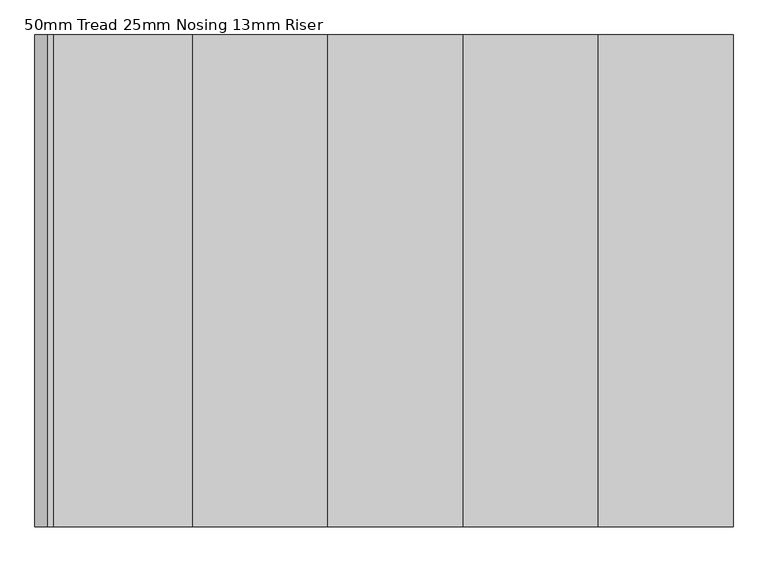
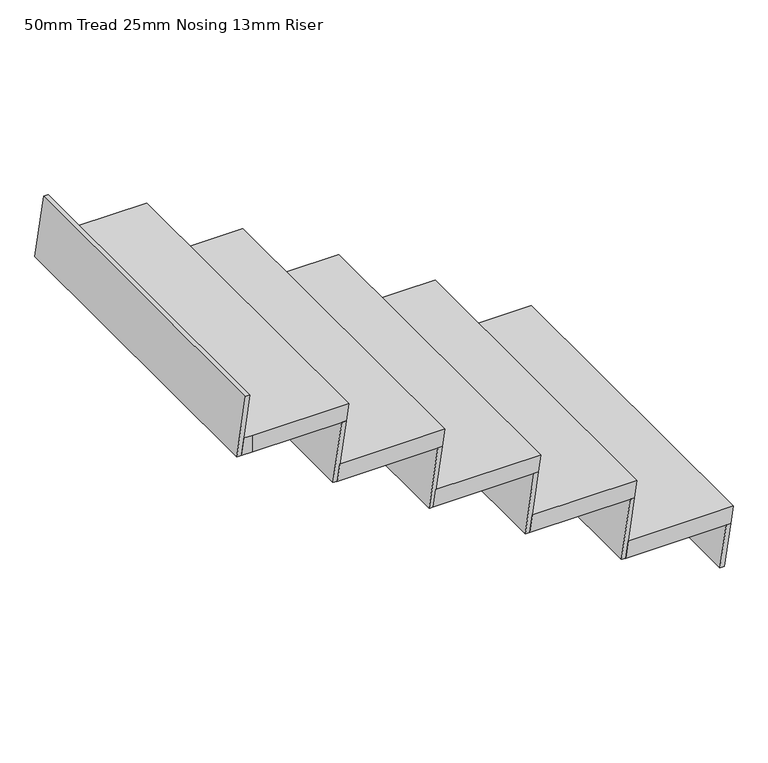
"""IFC4 building model written with IfcOpenShell, lengths in millimetres: stair flight geometry, 50mm Tread 25mm Nosing 13mm Riser."""

from ifc_helpers import new_model, si_unit, origin, place, context, project, spatial, faceted_brep, source, transform, mapped, element, save


def stair_flight_50mm_tread_25mm_nosing_13mm_riser_f2c6acf0(model_context):
    return source(origin(), model_context, "Body", "Brep", [
        faceted_brep([(-10889.1151057, 1847.9055917, 173.9130435), (-10896.3026057, 1847.9055917, 123.9130435), (-10896.3026057, 847.8798105, 123.9130435), (-10889.1151057, 847.8798105, 173.9130435), (-10589.1151057, 847.8798105, 173.9130435), (-10589.1151057, 1847.9055917, 173.9130435), (-10596.3026057, 1847.9055917, 123.9130435), (-10596.3026057, 847.8798105, 123.9130435)], [[[0, 1, 2, 3]], [[3, 4, 5, 0]], [[2, 1, 6, 7]], [[4, 3, 2, 7]], [[0, 5, 6, 1]], [[5, 4, 7, 6]]]),
        faceted_brep([(-10596.3026057, 1847.9055917, 123.9130435), (-10614.1151057, 1847.9055917, 0.0), (-10626.7435957, 1847.9055917, 0.0), (-10608.9310957, 1847.9055917, 123.9130435), (-10596.3026057, 847.8798105, 123.9130435), (-10608.9310957, 847.8798105, 123.9130435), (-10626.7435957, 847.8798105, 0.0), (-10614.1151057, 847.8798105, 0.0)], [[[0, 1, 2, 3]], [[4, 5, 6, 7]], [[1, 0, 4, 7]], [[2, 1, 7, 6]], [[3, 2, 6, 5]], [[0, 3, 5, 4]]]),
        faceted_brep([(-10871.3026057, 1847.9055917, 297.826087), (-10896.3026057, 1847.9055917, 123.9130435), (-10908.9310957, 1847.9055917, 123.9130435), (-10883.9310957, 1847.9055917, 297.826087), (-10871.3026057, 847.8798105, 297.826087), (-10883.9310957, 847.8798105, 297.826087), (-10908.9310957, 847.8798105, 123.9130435), (-10896.3026057, 847.8798105, 123.9130435)], [[[0, 1, 2, 3]], [[4, 5, 6, 7]], [[1, 0, 4, 7]], [[2, 1, 7, 6]], [[3, 2, 6, 5]], [[0, 3, 5, 4]]]),
        faceted_brep([(-11164.1151057, 847.8798105, 347.826087), (-10864.1151057, 847.8798105, 347.826087), (-10864.1151057, 1847.9055917, 347.826087), (-11164.1151057, 1847.9055917, 347.826087), (-11171.3026057, 847.8798105, 297.826087), (-11171.3026057, 1847.9055917, 297.826087), (-10871.3026057, 1847.9055917, 297.826087), (-10871.3026057, 847.8798105, 297.826087)], [[[0, 1, 2, 3]], [[4, 5, 6, 7]], [[1, 0, 4, 7]], [[3, 2, 6, 5]], [[3, 5, 4, 0]], [[2, 1, 7, 6]]]),
        faceted_brep([(-11146.3026057, 1847.9055917, 471.7391304), (-11171.3026057, 1847.9055917, 297.826087), (-11183.9310957, 1847.9055917, 297.826087), (-11158.9310957, 1847.9055917, 471.7391304), (-11146.3026057, 847.8798105, 471.7391304), (-11158.9310957, 847.8798105, 471.7391304), (-11183.9310957, 847.8798105, 297.826087), (-11171.3026057, 847.8798105, 297.826087)], [[[0, 1, 2, 3]], [[4, 5, 6, 7]], [[1, 0, 4, 7]], [[2, 1, 7, 6]], [[3, 2, 6, 5]], [[0, 3, 5, 4]]]),
        faceted_brep([(-11439.1151057, 847.8798105, 521.7391304), (-11139.1151057, 847.8798105, 521.7391304), (-11139.1151057, 1847.9055917, 521.7391304), (-11439.1151057, 1847.9055917, 521.7391304), (-11446.3026057, 847.8798105, 471.7391304), (-11446.3026057, 1847.9055917, 471.7391304), (-11146.3026057, 1847.9055917, 471.7391304), (-11146.3026057, 847.8798105, 471.7391304)], [[[0, 1, 2, 3]], [[4, 5, 6, 7]], [[1, 0, 4, 7]], [[3, 2, 6, 5]], [[3, 5, 4, 0]], [[2, 1, 7, 6]]]),
        faceted_brep([(-11421.3026057, 1847.9055917, 645.6521739), (-11446.3026057, 1847.9055917, 471.7391304), (-11458.9310957, 1847.9055917, 471.7391304), (-11433.9310957, 1847.9055917, 645.6521739), (-11421.3026057, 847.8798105, 645.6521739), (-11433.9310957, 847.8798105, 645.6521739), (-11458.9310957, 847.8798105, 471.7391304), (-11446.3026057, 847.8798105, 471.7391304)], [[[0, 1, 2, 3]], [[4, 5, 6, 7]], [[1, 0, 4, 7]], [[2, 1, 7, 6]], [[3, 2, 6, 5]], [[0, 3, 5, 4]]]),
        faceted_brep([(-11714.1151057, 847.8798105, 695.6521739), (-11414.1151057, 847.8798105, 695.6521739), (-11414.1151057, 1847.9055917, 695.6521739), (-11714.1151057, 1847.9055917, 695.6521739), (-11721.3026057, 847.8798105, 645.6521739), (-11721.3026057, 1847.9055917, 645.6521739), (-11421.3026057, 1847.9055917, 645.6521739), (-11421.3026057, 847.8798105, 645.6521739)], [[[0, 1, 2, 3]], [[4, 5, 6, 7]], [[1, 0, 4, 7]], [[3, 2, 6, 5]], [[3, 5, 4, 0]], [[2, 1, 7, 6]]]),
        faceted_brep([(-11971.3026057, 1847.9055917, 993.4782609), (-11996.3026057, 1847.9055917, 819.5652174), (-12008.9310957, 1847.9055917, 819.5652174), (-11983.9310957, 1847.9055917, 993.4782609), (-11971.3026057, 847.8798105, 993.4782609), (-11983.9310957, 847.8798105, 993.4782609), (-12008.9310957, 847.8798105, 819.5652174), (-11996.3026057, 847.8798105, 819.5652174)], [[[0, 1, 2, 3]], [[4, 5, 6, 7]], [[1, 0, 4, 7]], [[2, 1, 7, 6]], [[3, 2, 6, 5]], [[0, 3, 5, 4]]]),
        faceted_brep([(-11696.3026057, 1847.9055917, 819.5652174), (-11721.3026057, 1847.9055917, 645.6521739), (-11733.9310957, 1847.9055917, 645.6521739), (-11708.9310957, 1847.9055917, 819.5652174), (-11696.3026057, 847.8798105, 819.5652174), (-11708.9310957, 847.8798105, 819.5652174), (-11733.9310957, 847.8798105, 645.6521739), (-11721.3026057, 847.8798105, 645.6521739)], [[[0, 1, 2, 3]], [[4, 5, 6, 7]], [[1, 0, 4, 7]], [[2, 1, 7, 6]], [[3, 2, 6, 5]], [[0, 3, 5, 4]]]),
        faceted_brep([(-11989.1151057, 847.8798105, 869.5652174), (-11964.1151057, 847.8798105, 869.5652174), (-11689.1151057, 847.8798105, 869.5652174), (-11689.1151057, 1847.9055917, 869.5652174), (-11989.1151057, 1847.9055917, 869.5652174), (-11996.3026057, 847.8798105, 819.5652174), (-11996.3026057, 1847.9055917, 819.5652174), (-11696.3026057, 1847.9055917, 819.5652174), (-11696.3026057, 847.8798105, 819.5652174), (-11964.1151057, 847.8798105, 819.5652174)], [[[0, 1, 2, 3, 4]], [[5, 6, 7, 8, 9]], [[1, 0, 5, 9]], [[2, 1, 9, 8]], [[4, 3, 7, 6]], [[4, 6, 5, 0]], [[3, 2, 8, 7]]]),
    ])


if __name__ == "__main__":
    model = new_model("IFC4")
    model_context = context("Model", 3, world=origin())
    ifc_project = project(units=[si_unit("LENGTHUNIT", "METRE", prefix="MILLI")], contexts=[model_context])
    site = spatial("IfcSite", under=ifc_project)
    building = spatial("IfcBuilding", under=site)
    placement = place(None, origin())
    stair_flight_50mm_tread_25mm_nosing_13mm_riser_shape = stair_flight_50mm_tread_25mm_nosing_13mm_riser_f2c6acf0(model_context)
    element("IfcStairFlight", 1, ObjectType="50mm Tread 25mm Nosing 13mm Riser", at=placement, inside=building, context=model_context, shape_type="MappedRepresentation", body=[
        mapped(stair_flight_50mm_tread_25mm_nosing_13mm_riser_shape, transform((0.0, 0.0, 0.0), x_axis=(1.0, 0.0, 0.0), y_axis=(0.0, 1.0, 0.0), z_axis=(0.0, 0.0, 1.0))),
    ])
    save(model, "model.ifc")
